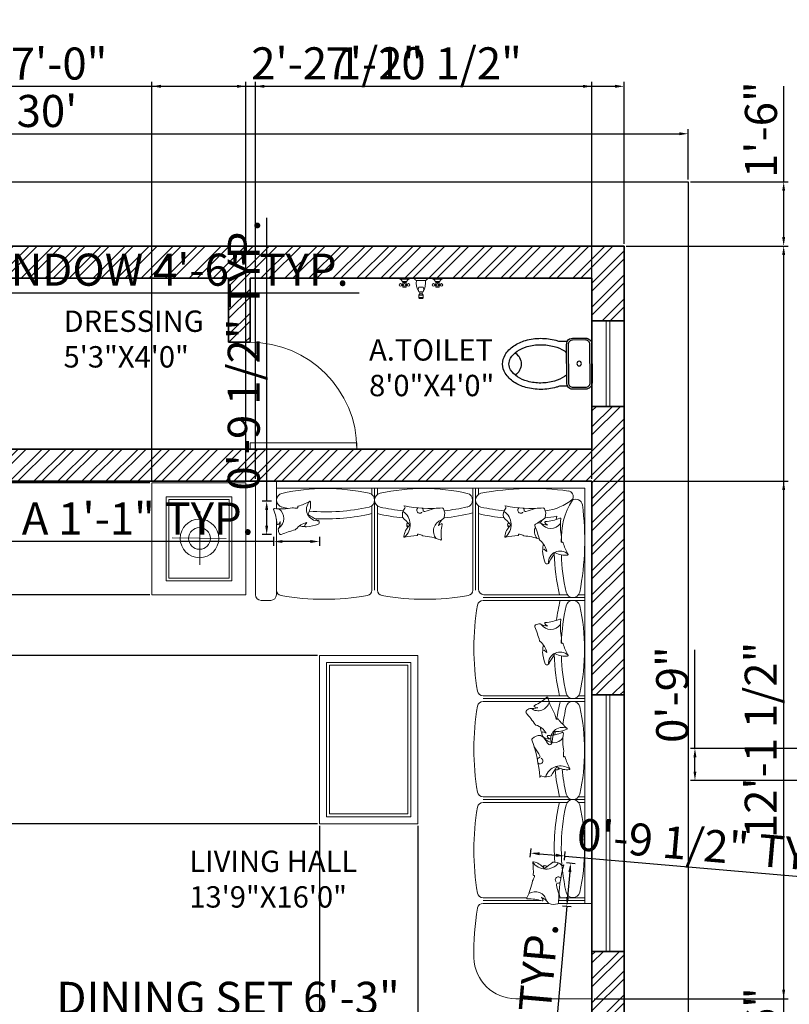
# Model space of a CAD drawing. Units: inches. Extents: x 638 to 1853, y 4393 to 5041.
# Tile 3 of 6: x 856 to 1072, y 4693 to 4970. Entities that reach past the tile are written whole.
import ezdxf

# ---------------------------------------------------------------- set-up
doc = ezdxf.new("R2010")
doc.units = ezdxf.units.IN
for name, color, linetype, lineweight in [('A-ANNO-DIMS', 2, 'Continuous', 18), ('A-AREA-IDEN', 7, 'Continuous', 18), ('A-DOOR', 4, 'Continuous', 18), ('A-FLOR-FIXT', 9, 'Continuous', 18), ('A-FURN', 26, 'Continuous', 13), ('A-GLAZ', 5, 'Continuous', 18), ('A-WALL', 7, 'Continuous', 35), ('A-WALL-PATT', 251, 'Continuous', 13), ('C-PROP', 7, 'Continuous', 25)]:
    doc.layers.add(name, color=color, linetype=linetype, lineweight=lineweight)
doc.layers.add('SANTEH', color=7, linetype='Continuous')
doc.styles.get("Standard").update_dxf_attribs({"font": 'arial.ttf'})
doc.dimstyles.new('ISO-25', dxfattribs={"dimtxt": 9, "dimasz": 2.5, "dimexe": 1.25, "dimexo": 0.625, "dimtad": 1, "dimdec": 1, "dimlunit": 3, "dimtxsty": 'Standard', "dimcen": 2.5, "dimadec": 0, "dimazin": 0, "dimtfac": 1, "dimtdec": 1, "dimtmove": 0, "dimatfit": 3, "dimfxl": 1, "dimarcsym": 0})

# ---------------------------------------------------------------- blocks, each defined once
blk = doc.blocks.new('*U3')
for p, q in [((-30, 0), (-30, -6)), ((0, 0), (0, -6))]:
    blk.add_line(p, q)
blk.add_lwpolyline([(0, 0), (0, 30), (-1.75, 30), (-1.75, 0)], close=True)
blk.add_arc((0, 0), 30, 90, 180)
blk = doc.blocks.new('K10-44')
at = {"layer": 'SANTEH'}
for points in [[(-182, 222.6, 0.020439), (-174, 197.6), (-174, 134.8, 0.262987), (-198.2, 92), (-198.2, -8, 0.414214), (-148.2, -58), (151.8, -58, 0.414214), (201.8, -8), (201.8, 92, 0.262987), (177.6, 134.8), (177.6, 197.6, 0.020439), (185.6, 222.6, 0.067459), (201.8, 342, 0.067459), (185.6, 461.3, 0.079812), (143.2, 554.1, 0.107118), (73.7, 621.5, 0.139889), (1.8, 642, 0.139889), (-70.1, 621.5, 0.107118), (-139.6, 554.1, 0.079812), (-182, 461.3, 0.067459), (-198.2, 342, 0.067459)], [(-148.2, 127), (151.8, 127, -0.414214), (186.8, 92), (186.8, -8, -0.414214), (151.8, -43), (-148.2, -43, -0.414214), (-183.2, -8), (-183.2, 92, -0.414214)]]:
    blk.add_lwpolyline(points, format="xyb", close=True, dxfattribs=at)
for points in [[(89.9, 142, 0.027307), (101.6, 157.6, 0.079812), (137.4, 235.9, 0.067459), (151.8, 342, 0.067459), (137.4, 448, 0.079812), (101.6, 526.4, 0.107118), (47.3, 579, 0.139889), (1.8, 592, 0.139889), (-43.7, 579, 0.107118), (-98, 526.4, 0.079812), (-133.8, 448, 0.067459), (-148.2, 342, 0.067459), (-133.8, 235.9, 0.079812), (-98, 157.6, 0.027307), (-86.4, 142, 0.139889)], [(-174, 134.8, -0.136371), (-148.2, 142), (151.8, 142, -0.136371), (177.6, 134.8)]]:
    blk.add_lwpolyline(points, format="xyb", dxfattribs=at)
blk.add_circle((1.8, 42), 18.3, dxfattribs=at)
blk.add_arc((1.8, 601.6), 105.3, 213.89944, 326.10056, dxfattribs=at)
blk = doc.blocks.new('Faucet - Bathroom front')
for p, q in [((-0.5, 4.25), (0.5, 4.25)), ((0.5, 3.75), (-0.5, 3.75)), ((-0.5, 3), (0.5, 3)), ((-0.25, 3), (-0.25, 3.5)), ((0.25, 3.5), (0.25, 3)), ((-5, 0), (-2.25, 0)), ((-4.5087, 0.25), (-2.7408, 0.25)), ((-4, 1.625), (-4.25, 1.625)), ((-4, 1.375), (-4.25, 1.375)), ((-3.1442, 0.75), (-4.0979, 0.75)), ((-3.25, 1.625), (-3, 1.625)), ((-3.25, 1.375), (-3, 1.375)), ((-1.5, 0), (1.5, 0)), ((-1, 0.5), (1, 0.5)), ((0.5, 2), (-0.5, 2)), ((2.25, 0), (5, 0)), ((2.7413, 0.25), (4.5092, 0.25)), ((3.25, 1.625), (3, 1.625)), ((3.25, 1.375), (3, 1.375)), ((4.1058, 0.75), (3.1521, 0.75)), ((4, 1.625), (4.25, 1.625)), ((4, 1.375), (4.25, 1.375))]:
    blk.add_line(p, q)
for points in [[(-0.25, 4.5), (0.25, 4.5)], [(-0.5, 3.75), (-0.5, 4.25)], [(0.25, 3.5), (-0.25, 3.5)], [(0.5, 4.25), (0.5, 3.75)]]:
    blk.add_lwpolyline(points)
for points in [[(-4, 1), (-4, 2), (-3.25, 2), (-3.25, 1)], [(3.25, 1), (3.25, 2), (4, 2), (4, 1)]]:
    blk.add_lwpolyline(points, close=True)
for centre in [(-4.5, 1.5), (-3.625, 1.5), (-2.75, 1.5), (2.75, 1.5), (3.625, 1.5), (4.5, 1.5)]:
    blk.add_circle(centre, 0.2795)
for centre, radius, start, end in [((-0.2575, 4.2575), 0.2426, 88.22243, 181.7776), ((0.2575, 4.2575), 0.2426, 358.2224, 91.77757), ((3, 1), 4.0311, 150.2551, 187.125), ((0.6413, 2.5), 1.246, 156.3417, 203.6583), ((-0.2575, 3.7425), 0.2426, 178.2224, 271.7776), ((0.2575, 3.7425), 0.2426, 268.2224, 1.777565), ((-3, 1), 4.0311, 352.875, 29.74488), ((-0.6413, 2.5), 1.246, 336.3417, 23.65835), ((-5.375, 1.375), 1.4252, 285.2551, 344.7449), ((-1.875, 1.375), 1.4252, 195.2551, 254.7449), ((-0.7962, -0.2038), 0.7327, 106.1502, 163.8498), ((0.7962, -0.2038), 0.7327, 16.1502, 73.84979), ((1.875, 1.375), 1.4252, 285.2551, 344.7449), ((5.375, 1.375), 1.4252, 195.2551, 254.7449)]:
    blk.add_arc(centre, radius, start, end)
blk = doc.blocks.new('*D16')
at = {"layer": 'A-ANNO-DIMS', "color": 0, "lineweight": -2, "transparency": 16777216}
for p, q in [((683.34, 4924.82), (683.34, 4938.95)), ((1043.34, 4924.82), (1043.34, 4938.95)), ((685.84, 4937.7), (1040.84, 4937.7))]:
    blk.add_line(p, q, dxfattribs=at)
at = {"layer": 'A-ANNO-DIMS', "color": 0, "transparency": 16777216}
for points in [[(685.84, 4938.12), (685.84, 4937.29), (683.34, 4937.7)], [(1040.84, 4938.12), (1040.84, 4937.29), (1043.34, 4937.7)]]:
    blk.add_solid(points, dxfattribs=at)
at = {"layer": 'Defpoints', "color": 0, "transparency": 16777216}
for p in [(1043.34, 4937.7), (683.34, 4924.19), (1043.34, 4924.19)]:
    blk.add_point(p, dxfattribs=at)
at = {"layer": 'A-ANNO-DIMS', "color": 0, "transparency": 16777216, "insert": (863.34, 4942.93), "char_height": 9, "attachment_point": 5}
blk.add_mtext("30'", dxfattribs=at)
blk = doc.blocks.new('SOFA-THROW-PILLOW-A')
for centre, radius, start, end in [((0.39, 10.82), 0.394, 117.1304, 200.9482), ((1.62, 8.42), 3.09, 92.7962, 117.1304), ((3.55, 15.03), 4.09, 239.5087, 271.0429), ((4.49, 13.18), 3.27, 214.0212, 325.1506), ((2.96, 11.66), 0.197, 93.9947, 209.557), ((3.91, 12.2), 1.3, 209.557, 257.0475), ((2.03, 24.94), 13.11, 273.9947, 292.2174), ((7.06, 12.62), 0.197, 353.9832, 112.2174), ((23.64, 10.87), 16.48, 173.9832, 191.5286), ((-38.21, -3.96), 40.94, 15.1521, 20.9482), ((1.69, 6.84), 0.394, 195.1521, 232.4345), ((-1.66, 2.48), 5.11, 10.921, 52.4345), ((10.08, 4.04), 7.86, 168.5381, 180.9308), ((15.26, 6.3), 7.86, 170.6752, 180.5669), ((7.59, 6.23), 0.197, 180.5669, 291.9475), ((7.74, 5.86), 0.197, 17.478, 111.9475), ((23.64, 10.87), 16.48, 197.478, 209.4698), ((2.54, 3.69), 0.394, 41.4659, 190.4525), ((16.93, 5.2), 14.87, 186.1256, 199.3393), ((6.12, 6.85), 4.39, 221.4659, 230.8131), ((7.05, 0.33), 3.25, 45.6927, 183.5175), ((38.1, -18.02), 38.77, 147.1103, 151.1368), ((5.7, 2.93), 0.197, 60.4242, 147.1103), ((8.39, 7.66), 5.25, 240.4242, 278.3824), ((3.28, 0.41), 0.394, 199.3393, 253.8009), ((3.38, 0.76), 0.764, 253.8009, 355.0524), ((9.13, 2.67), 0.197, 278.3824, 29.4698)]:
    blk.add_arc(centre, radius, start, end)
blk = doc.blocks.new('SOFA-THROW-PILLOW-B')
for centre, radius, start, end in [((3.19, 7), 3.19, 142.1663, 190.7613), ((0.36, 9.2), 0.394, 322.1663, 79.3422), ((8, 49.83), 40.94, 259.5852, 274.4465), ((4.89, 8.38), 0.833, 127.3565, 320.7762), ((4.94, 8.37), 0.873, 7.7015, 42.1556), ((5.42, 8.43), 0.394, 357.6426, 7.7015), ((6.2, 8.4), 0.394, 177.6426, 284.049), ((1.87, 25.7), 18.23, 284.049, 292.3823), ((9, 8.5), 0.394, 91.386, 118.7955), ((8, 49.83), 40.94, 271.386, 274.4465), ((11.21, 8.61), 0.394, 26.666, 94.4465), ((8.69, 7.35), 3.21, 342.3377, 26.666), ((-27.35, -21.02), 38.77, 40.8329, 45.0245), ((-2.23, 4.27), 4.44, 308.8947, 57.3952), ((12.01, 2.51), 3.27, 107.7628, 218.8922), ((14.05, 2.89), 4.09, 126.6071, 164.7845), ((11.38, 6.49), 0.394, 306.6071, 342.3377), ((5.62, 0.31), 5.25, 134.9211, 172.124), ((2, 4.24), 0.787, 127.662, 234.1573), ((15.2, 45.86), 44.04, 251.4982, 252.2888), ((7.81, -38.62), 44.04, 97.7018, 97.7206), ((1.84, 4.2), 0.197, 293.8315, 40.8329), ((11.24, 3.33), 1.3, 103.2985, 150.7891), ((23.99, 1.58), 13.11, 167.7363, 185.959), ((10.98, 4.41), 0.197, 347.7363, 103.2985), ((0.62, 1), 0.197, 172.124, 283.2114), ((0.62, 1), 0.197, 172.124, 283.2114), ((4.43, -15.23), 16.48, 91.2196, 103.2114), ((4.08, 1.44), 0.197, 271.2196, 5.689), ((4.47, 1.48), 0.197, 74.3085, 185.689), ((2.4, -5.9), 7.86, 64.4168, 74.3085), ((4.43, -15.23), 16.48, 67.7248, 85.2702), ((10.75, 0.2), 0.197, 247.7248, 5.959)]:
    blk.add_arc(centre, radius, start, end)
blk = doc.blocks.new('WINDOW-GLAZING-24IN')
for p, q in [((0, 24), (0, 0)), ((1, 24), (1, 0))]:
    blk.add_line(p, q)
blk = doc.blocks.new('WINDOW-GLAZING-72IN')
for p, q in [((0, 72), (0, 0)), ((1, 72), (1, 0))]:
    blk.add_line(p, q)
blk = doc.blocks.new('*D44')
at = {"layer": 'A-ANNO-DIMS', "color": 0, "lineweight": -2, "transparency": 16777216}
for p, q in [((926.95, 4823.26), (805.91, 4823.26)), ((926.95, 4824.56), (926.95, 4822.01)), ((937.31, 4823.26), (929.45, 4823.26)), ((939.81, 4824.56), (939.81, 4822.01))]:
    blk.add_line(p, q, dxfattribs=at)
at = {"layer": 'A-ANNO-DIMS', "color": 0, "transparency": 16777216}
for points in [[(929.45, 4823.67), (929.45, 4822.84), (926.95, 4823.26)], [(937.31, 4823.67), (937.31, 4822.84), (939.81, 4823.26)]]:
    blk.add_solid(points, dxfattribs=at)
at = {"layer": 'Defpoints', "color": 0, "transparency": 16777216}
for p in [(926.95, 4825.19), (926.95, 4823.26), (939.81, 4825.19)]:
    blk.add_point(p, dxfattribs=at)
at = {"layer": 'A-ANNO-DIMS', "color": 0, "transparency": 16777216, "insert": (865.18, 4828.54), "char_height": 9, "attachment_point": 5}
blk.add_mtext('PILLOW A 1\'-1" TYP.', dxfattribs=at)
blk = doc.blocks.new('*D45')
at = {"layer": 'A-ANNO-DIMS', "color": 0, "lineweight": -2, "transparency": 16777216}
for p, q in [((925.02, 4834.56), (925.02, 4914.14)), ((926.33, 4834.56), (923.77, 4834.56)), ((925.02, 4827.69), (925.02, 4832.06)), ((926.33, 4825.19), (923.77, 4825.19))]:
    blk.add_line(p, q, dxfattribs=at)
at = {"layer": 'A-ANNO-DIMS', "color": 0, "transparency": 16777216}
for points in [[(924.61, 4832.06), (925.44, 4832.06), (925.02, 4834.56)], [(924.61, 4827.69), (925.44, 4827.69), (925.02, 4825.19)]]:
    blk.add_solid(points, dxfattribs=at)
at = {"layer": 'Defpoints', "color": 0, "transparency": 16777216}
for p in [(925.02, 4834.56), (926.95, 4834.56), (926.95, 4825.19)]:
    blk.add_point(p, dxfattribs=at)
at = {"layer": 'A-ANNO-DIMS', "color": 0, "transparency": 16777216, "insert": (919.75, 4875.6), "char_height": 9, "attachment_point": 5, "rotation": 90}
blk.add_mtext('0\'-9 1/2" TYP.', dxfattribs=at)
blk = doc.blocks.new('*D46')
at = {"layer": 'A-ANNO-DIMS', "color": 0, "lineweight": -2, "transparency": 16777216}
for p, q in [((779.34, 4900.57), (779.34, 4891.84)), ((833.34, 4900.57), (833.34, 4891.84)), ((781.84, 4893.09), (830.84, 4893.09)), ((833.34, 4893.09), (950.98, 4893.09))]:
    blk.add_line(p, q, dxfattribs=at)
at = {"layer": 'A-ANNO-DIMS', "color": 0, "transparency": 16777216}
for points in [[(781.84, 4893.51), (781.84, 4892.68), (779.34, 4893.09)], [(830.84, 4893.51), (830.84, 4892.68), (833.34, 4893.09)]]:
    blk.add_solid(points, dxfattribs=at)
at = {"layer": 'Defpoints', "color": 0, "transparency": 16777216}
for p in [(779.34, 4901.19), (833.34, 4901.19), (833.34, 4893.09)]:
    blk.add_point(p, dxfattribs=at)
at = {"layer": 'A-ANNO-DIMS', "color": 0, "transparency": 16777216, "insert": (893.41, 4898.38), "char_height": 9, "attachment_point": 5}
blk.add_mtext('WINDOW 4\'-6" TYP.', dxfattribs=at)
blk = doc.blocks.new('*D50')
at = {"layer": 'A-ANNO-DIMS', "color": 0, "lineweight": -2, "transparency": 16777216}
for p, q in [((1009.16, 4733.11), (1011.59, 4732.9)), ((1010.13, 4730.52), (1009.51, 4723.42)), ((1009.29, 4720.93), (998.74, 4600.35)), ((1008.1, 4721.03), (1010.54, 4720.82))]:
    blk.add_line(p, q, dxfattribs=at)
at = {"layer": 'A-ANNO-DIMS', "color": 0, "transparency": 16777216}
for points in [[(1009.71, 4730.55), (1010.54, 4730.48), (1010.35, 4733.01)], [(1009.09, 4723.46), (1009.92, 4723.38), (1009.29, 4720.93)]]:
    blk.add_solid(points, dxfattribs=at)
at = {"layer": 'Defpoints', "color": 0, "transparency": 16777216}
for p in [(1008.54, 4733.16), (1007.48, 4721.09), (1009.29, 4720.93)]:
    blk.add_point(p, dxfattribs=at)
at = {"layer": 'A-ANNO-DIMS', "color": 0, "transparency": 16777216, "insert": (998.65, 4659.85), "char_height": 9, "attachment_point": 5, "rotation": 85}
blk.add_mtext('PILLOW B 1\'-0" TYP.', dxfattribs=at)
blk = doc.blocks.new('*D51')
at = {"layer": 'A-ANNO-DIMS', "color": 0, "lineweight": -2, "transparency": 16777216}
for p, q in [((999.03, 4734.62), (999.24, 4737.06)), ((1001.62, 4735.59), (1006.2, 4735.19)), ((1008.59, 4733.79), (1008.8, 4736.22)), ((1008.69, 4734.98), (1087.97, 4728.04))]:
    blk.add_line(p, q, dxfattribs=at)
at = {"layer": 'A-ANNO-DIMS', "color": 0, "transparency": 16777216}
for points in [[(1001.66, 4736.01), (1001.59, 4735.18), (999.13, 4735.81)], [(1006.24, 4735.61), (1006.17, 4734.78), (1008.69, 4734.98)]]:
    blk.add_solid(points, dxfattribs=at)
at = {"layer": 'Defpoints', "color": 0, "transparency": 16777216}
for p in [(1008.69, 4734.98), (998.97, 4734), (1008.54, 4733.16)]:
    blk.add_point(p, dxfattribs=at)
at = {"layer": 'A-ANNO-DIMS', "color": 0, "transparency": 16777216, "insert": (1050.04, 4736.66), "char_height": 9, "attachment_point": 5, "rotation": 355}
blk.add_mtext('0\'-9 1/2" TYP.', dxfattribs=at)
blk = doc.blocks.new('*D62')
at = {"layer": 'A-ANNO-DIMS', "color": 0, "lineweight": -2, "transparency": 16777216}
for p, q in [((786.73, 4678.11), (786.73, 4689.96)), ((861.6, 4678.11), (861.6, 4689.96)), ((789.23, 4688.71), (859.1, 4688.71)), ((861.6, 4688.71), (964.27, 4688.71))]:
    blk.add_line(p, q, dxfattribs=at)
at = {"layer": 'A-ANNO-DIMS', "color": 0, "transparency": 16777216}
for points in [[(789.23, 4689.13), (789.23, 4688.3), (786.73, 4688.71)], [(859.1, 4689.13), (859.1, 4688.3), (861.6, 4688.71)]]:
    blk.add_solid(points, dxfattribs=at)
at = {"layer": 'Defpoints', "color": 0, "transparency": 16777216}
for p in [(861.6, 4688.71), (786.73, 4677.48), (861.6, 4677.48)]:
    blk.add_point(p, dxfattribs=at)
at = {"layer": 'A-ANNO-DIMS', "color": 0, "transparency": 16777216, "insert": (914.18, 4694), "char_height": 9, "attachment_point": 5}
blk.add_mtext('DINING SET 6\'-3"', dxfattribs=at)
blk = doc.blocks.new('*D74')
at = {"layer": 'A-ANNO-DIMS', "color": 0, "lineweight": -2, "transparency": 16777216}
for p, q in [((701.34, 4906.82), (701.34, 4952.27)), ((703.84, 4951.02), (1022.84, 4951.02)), ((1025.34, 4906.82), (1025.34, 4952.27))]:
    blk.add_line(p, q, dxfattribs=at)
at = {"layer": 'A-ANNO-DIMS', "color": 0, "transparency": 16777216}
for points in [[(703.84, 4951.44), (703.84, 4950.6), (701.34, 4951.02)], [(1022.84, 4951.44), (1022.84, 4950.6), (1025.34, 4951.02)]]:
    blk.add_solid(points, dxfattribs=at)
at = {"layer": 'Defpoints', "color": 0, "transparency": 16777216}
for p in [(1025.34, 4951.02), (701.34, 4906.19), (1025.34, 4906.19)]:
    blk.add_point(p, dxfattribs=at)
at = {"layer": 'A-ANNO-DIMS', "color": 0, "transparency": 16777216, "insert": (863.34, 4956.24), "char_height": 9, "attachment_point": 5}
blk.add_mtext('27\'-0"', dxfattribs=at)
blk = doc.blocks.new('*D75')
at = {"layer": 'A-ANNO-DIMS', "color": 0, "lineweight": -2, "transparency": 16777216}
for p, q in [((1025.97, 4906.19), (1071.42, 4906.19)), ((1070.17, 4458.69), (1070.17, 4903.69)), ((896.97, 4456.19), (1071.42, 4456.19))]:
    blk.add_line(p, q, dxfattribs=at)
at = {"layer": 'A-ANNO-DIMS', "color": 0, "transparency": 16777216}
for points in [[(1069.75, 4903.69), (1070.58, 4903.69), (1070.17, 4906.19)], [(1069.75, 4458.69), (1070.58, 4458.69), (1070.17, 4456.19)]]:
    blk.add_solid(points, dxfattribs=at)
at = {"layer": 'Defpoints', "color": 0, "transparency": 16777216}
for p in [(1025.34, 4906.19), (1070.17, 4906.19), (896.34, 4456.19)]:
    blk.add_point(p, dxfattribs=at)
at = {"layer": 'A-ANNO-DIMS', "color": 0, "transparency": 16777216, "insert": (1064.94, 4681.19), "char_height": 9, "attachment_point": 5, "rotation": 90}
blk.add_mtext('37\'-6"', dxfattribs=at)
blk = doc.blocks.new('*D77')
at = {"layer": 'A-ANNO-DIMS', "color": 0, "lineweight": -2, "transparency": 16777216}
for p, q in [((1070.17, 4924.19), (1070.17, 4951.02)), ((1043.97, 4924.19), (1071.42, 4924.19)), ((1070.17, 4908.69), (1070.17, 4921.69)), ((1025.97, 4906.19), (1071.42, 4906.19))]:
    blk.add_line(p, q, dxfattribs=at)
at = {"layer": 'A-ANNO-DIMS', "color": 0, "transparency": 16777216}
for points in [[(1069.75, 4921.69), (1070.58, 4921.69), (1070.17, 4924.19)], [(1069.75, 4908.69), (1070.58, 4908.69), (1070.17, 4906.19)]]:
    blk.add_solid(points, dxfattribs=at)
at = {"layer": 'Defpoints', "color": 0, "transparency": 16777216}
for p in [(1043.34, 4924.19), (1070.17, 4924.19), (1025.34, 4906.19)]:
    blk.add_point(p, dxfattribs=at)
at = {"layer": 'A-ANNO-DIMS', "color": 0, "transparency": 16777216, "insert": (1064.95, 4938.86), "char_height": 9, "attachment_point": 5, "rotation": 90}
blk.add_mtext('1\'-6"', dxfattribs=at)
blk = doc.blocks.new('*D82')
at = {"layer": 'A-ANNO-DIMS', "color": 0, "lineweight": -2, "transparency": 16777216}
for p, q in [((921.85, 4840.82), (921.85, 4952.27)), ((924.35, 4951.02), (1013.84, 4951.02)), ((1016.34, 4840.82), (1016.34, 4952.27))]:
    blk.add_line(p, q, dxfattribs=at)
at = {"layer": 'A-ANNO-DIMS', "color": 0, "transparency": 16777216}
for points in [[(924.35, 4951.44), (924.35, 4950.6), (921.85, 4951.02)], [(1013.84, 4951.44), (1013.84, 4950.6), (1016.34, 4951.02)]]:
    blk.add_solid(points, dxfattribs=at)
at = {"layer": 'Defpoints', "color": 0, "transparency": 16777216}
for p in [(1016.34, 4951.02), (921.85, 4840.19), (1016.34, 4840.19)]:
    blk.add_point(p, dxfattribs=at)
at = {"layer": 'A-ANNO-DIMS', "color": 0, "transparency": 16777216, "insert": (969.1, 4956.3), "char_height": 9, "attachment_point": 5}
blk.add_mtext('7\'-10 1/2"', dxfattribs=at)
blk = doc.blocks.new('*D83')
at = {"layer": 'A-ANNO-DIMS', "color": 0, "lineweight": -2, "transparency": 16777216}
for p, q in [((1016.97, 4840.19), (1071.42, 4840.19)), ((1070.17, 4697.42), (1070.17, 4837.69)), ((1016.97, 4694.92), (1071.42, 4694.92))]:
    blk.add_line(p, q, dxfattribs=at)
at = {"layer": 'A-ANNO-DIMS', "color": 0, "transparency": 16777216}
for points in [[(1069.75, 4837.69), (1070.58, 4837.69), (1070.17, 4840.19)], [(1069.75, 4697.42), (1070.58, 4697.42), (1070.17, 4694.92)]]:
    blk.add_solid(points, dxfattribs=at)
at = {"layer": 'Defpoints', "color": 0, "transparency": 16777216}
for p in [(1016.34, 4840.19), (1070.17, 4840.19), (1016.34, 4694.92)]:
    blk.add_point(p, dxfattribs=at)
at = {"layer": 'A-ANNO-DIMS', "color": 0, "transparency": 16777216, "insert": (1064.89, 4767.56), "char_height": 9, "attachment_point": 5, "rotation": 90}
blk.add_mtext('12\'-1 1/2"', dxfattribs=at)
blk = doc.blocks.new('*D84')
at = {"layer": 'A-ANNO-DIMS', "color": 0, "lineweight": -2, "transparency": 16777216}
for p, q in [((939.87, 4743.42), (939.87, 4416.12)), ((967.43, 4743.42), (967.43, 4416.12)), ((942.37, 4417.37), (964.93, 4417.37)), ((967.43, 4417.37), (1016.23, 4417.37))]:
    blk.add_line(p, q, dxfattribs=at)
at = {"layer": 'A-ANNO-DIMS', "color": 0, "transparency": 16777216}
for points in [[(942.37, 4417.79), (942.37, 4416.95), (939.87, 4417.37)], [(964.93, 4417.79), (964.93, 4416.95), (967.43, 4417.37)]]:
    blk.add_solid(points, dxfattribs=at)
at = {"layer": 'Defpoints', "color": 0, "transparency": 16777216}
for p in [(939.87, 4744.04), (967.43, 4744.04), (967.43, 4417.37)]:
    blk.add_point(p, dxfattribs=at)
at = {"layer": 'A-ANNO-DIMS', "color": 0, "transparency": 16777216, "insert": (993.08, 4422.65), "char_height": 9, "attachment_point": 5}
blk.add_mtext('2\'-3 1/2"', dxfattribs=at)
blk = doc.blocks.new('*D85')
at = {"layer": 'A-ANNO-DIMS', "color": 0, "lineweight": -2, "transparency": 16777216}
for p, q in [((939.25, 4791.29), (655.27, 4791.29)), ((656.52, 4746.54), (656.52, 4788.79)), ((939.25, 4744.04), (655.27, 4744.04))]:
    blk.add_line(p, q, dxfattribs=at)
at = {"layer": 'A-ANNO-DIMS', "color": 0, "transparency": 16777216}
for points in [[(656.1, 4788.79), (656.93, 4788.79), (656.52, 4791.29)], [(656.1, 4746.54), (656.93, 4746.54), (656.52, 4744.04)]]:
    blk.add_solid(points, dxfattribs=at)
at = {"layer": 'Defpoints', "color": 0, "transparency": 16777216}
for p in [(656.52, 4791.29), (939.87, 4791.29), (939.87, 4744.04)]:
    blk.add_point(p, dxfattribs=at)
at = {"layer": 'A-ANNO-DIMS', "color": 0, "transparency": 16777216, "insert": (651.29, 4767.66), "char_height": 9, "attachment_point": 5, "rotation": 90}
blk.add_mtext('3\'-11"', dxfattribs=at)
blk = doc.blocks.new('*D86')
at = {"layer": 'A-ANNO-DIMS', "color": 0, "lineweight": -2, "transparency": 16777216}
for p, q in [((892.82, 4840.37), (892.82, 4952.27)), ((895.32, 4951.02), (916.69, 4951.02)), ((919.19, 4840.37), (919.19, 4952.27)), ((919.19, 4951.02), (967.99, 4951.02))]:
    blk.add_line(p, q, dxfattribs=at)
at = {"layer": 'A-ANNO-DIMS', "color": 0, "transparency": 16777216}
for points in [[(895.32, 4951.44), (895.32, 4950.6), (892.82, 4951.02)], [(916.69, 4951.44), (916.69, 4950.6), (919.19, 4951.02)]]:
    blk.add_solid(points, dxfattribs=at)
at = {"layer": 'Defpoints', "color": 0, "transparency": 16777216}
for p in [(919.19, 4951.02), (892.82, 4839.74), (919.19, 4839.74)]:
    blk.add_point(p, dxfattribs=at)
at = {"layer": 'A-ANNO-DIMS', "color": 0, "transparency": 16777216, "insert": (944.84, 4956.3), "char_height": 9, "attachment_point": 5}
blk.add_mtext('2\'-2 1/2"', dxfattribs=at)
blk = doc.blocks.new('*D87')
at = {"layer": 'A-ANNO-DIMS', "color": 0, "lineweight": -2, "transparency": 16777216}
for p, q in [((656.52, 4839.74), (656.52, 4888.54)), ((892.19, 4839.74), (655.27, 4839.74)), ((656.52, 4810.75), (656.52, 4837.24)), ((892.19, 4808.25), (655.27, 4808.25))]:
    blk.add_line(p, q, dxfattribs=at)
at = {"layer": 'A-ANNO-DIMS', "color": 0, "transparency": 16777216}
for points in [[(656.1, 4837.24), (656.93, 4837.24), (656.52, 4839.74)], [(656.1, 4810.75), (656.93, 4810.75), (656.52, 4808.25)]]:
    blk.add_solid(points, dxfattribs=at)
at = {"layer": 'Defpoints', "color": 0, "transparency": 16777216}
for p in [(656.52, 4839.74), (892.82, 4839.74), (892.82, 4808.25)]:
    blk.add_point(p, dxfattribs=at)
at = {"layer": 'A-ANNO-DIMS', "color": 0, "transparency": 16777216, "insert": (651.24, 4865.39), "char_height": 9, "attachment_point": 5, "rotation": 90}
blk.add_mtext('2\'-7 1/2"', dxfattribs=at)
blk = doc.blocks.new('*D93')
at = {"layer": 'A-ANNO-DIMS', "color": 0, "lineweight": -2, "transparency": 16777216}
for p, q in [((1045.26, 4765.19), (1045.26, 4792.87)), ((1284.46, 4765.19), (1044.01, 4765.19)), ((1045.26, 4758.69), (1045.26, 4762.69)), ((1275.46, 4756.19), (1044.01, 4756.19))]:
    blk.add_line(p, q, dxfattribs=at)
at = {"layer": 'A-ANNO-DIMS', "color": 0, "transparency": 16777216}
for points in [[(1044.84, 4762.69), (1045.67, 4762.69), (1045.26, 4765.19)], [(1044.84, 4758.69), (1045.67, 4758.69), (1045.26, 4756.19)]]:
    blk.add_solid(points, dxfattribs=at)
at = {"layer": 'Defpoints', "color": 0, "transparency": 16777216}
for p in [(1045.26, 4765.19), (1285.08, 4765.19), (1276.08, 4756.19)]:
    blk.add_point(p, dxfattribs=at)
at = {"layer": 'A-ANNO-DIMS', "color": 0, "transparency": 16777216, "insert": (1040.04, 4780.28), "char_height": 9, "attachment_point": 5, "rotation": 90}
blk.add_mtext('0\'-9"', dxfattribs=at)

msp = doc.modelspace()

# ---------------------------------------------------------------- hatches: boundary and pattern name
at = {"layer": 'A-WALL-PATT', "transparency": 33554687}
h = msp.add_hatch(dxfattribs=at)
h.set_pattern_fill('ANSI32', color=256, scale=0.5)
h.paths.add_polyline_path([(779.34, 4906.19), (701.34, 4906.19), (701.34, 4531.19), (710.34, 4531.19), (710.34, 4561.19), (758.34, 4561.19), (758.34, 4528.19), (764.34, 4528.19), (767.34, 4528.19), (767.34, 4561.19), (821.34, 4561.19), (821.34, 4570.19), (710.34, 4570.19), (710.34, 4756.19), (767.34, 4756.19), (767.34, 4702.19), (791.34, 4702.19), (791.34, 4708.19), (773.34, 4708.19), (773.34, 4756.19), (845.34, 4756.19), (845.34, 4708.19), (827.35, 4708.19), (827.35, 4705.02), (827.34, 4702.19), (851.34, 4702.19), (851.34, 4771.19), (845.34, 4771.19), (842.34, 4771.19), (842.34, 4765.19), (710.34, 4765.19), (710.34, 4897.19), (779.34, 4897.19)])
h.paths.add_polyline_path([(1025.34, 4906.19), (833.34, 4906.19), (833.34, 4897.19), (842.34, 4897.19), (842.34, 4882.21), (842.34, 4879.19), (851.34, 4879.19), (851.34, 4897.19), (914.34, 4897.19), (914.34, 4879.19), (920.34, 4879.19), (920.34, 4897.19), (1016.34, 4897.19), (1016.34, 4885.19), (1025.34, 4885.19)])
h.paths.add_polyline_path([(851.34, 4840.19), (1016.34, 4840.19), (1016.34, 4780.19), (1025.34, 4780.19), (1025.34, 4861.19), (1016.34, 4861.19), (1016.34, 4849.19), (842.34, 4849.19), (842.34, 4807.19), (851.34, 4807.19)])
h.paths.add_polyline_path([(1025.34, 4708.19), (1016.34, 4708.19), (1016.34, 4694.92), (1016.34, 4648.19), (996.84, 4648.19), (996.84, 4639.19), (1025.34, 4639.19)])
h.paths.add_polyline_path([(972.84, 4648.19), (944.34, 4648.19), (944.34, 4561.19), (953.34, 4561.19), (953.34, 4639.19), (972.84, 4639.19)])
h.paths.add_polyline_path([(896.34, 4648.19), (887.34, 4648.19), (887.34, 4570.19), (863.34, 4570.19), (863.34, 4561.19), (887.34, 4561.19), (887.34, 4552.19), (896.34, 4552.19), (896.34, 4561.19), (904.34, 4561.19), (904.34, 4567.19), (904.34, 4570.19), (896.34, 4570.19)])
h.paths.add_polyline_path([(896.34, 4504.19), (887.34, 4504.19), (887.34, 4465.19), (839.34, 4465.19), (839.34, 4456.19), (896.34, 4456.19)])
h.paths.add_polyline_path([(779.34, 4465.19), (767.34, 4465.19), (767.34, 4498.19), (758.34, 4498.19), (758.34, 4465.19), (710.34, 4465.19), (710.34, 4495.19), (701.34, 4495.19), (701.34, 4456.19), (779.34, 4456.19)])
h.paths.add_polyline_path([(865.86, 4868.68), (912.64, 4868.68), (912.64, 4891.07), (865.86, 4891.07)], flags=9)
h.paths.add_polyline_path([(730.31, 4828.82), (807.82, 4828.82), (807.82, 4851.21), (730.31, 4851.21)], flags=25)

# ---------------------------------------------------------------- linework, layer by layer
at = {"layer": 'A-FURN'}
for p, q in [((921.85, 4840.19), (1016.34, 4840.19)), ((921.85, 4840.19), (921.85, 4808.31)), ((927.76, 4840.19), (927.76, 4832.44)), ((1016.34, 4694.92), (1016.34, 4840.19)), ((927.76, 4838.23), (1014.37, 4838.23)), ((954.53, 4838.23), (954.53, 4836.47)), ((955.32, 4838.23), (955.32, 4809.62)), ((956.1, 4838.23), (956.1, 4836.47)), ((982.88, 4838.23), (982.88, 4809.62)), ((983.66, 4838.23), (983.66, 4809.62)), ((984.45, 4838.23), (984.45, 4836.44)), ((1014.37, 4721.69), (1014.37, 4838.23)), ((906.24, 4831.76), (906.24, 4816.75)), ((954.53, 4833.24), (954.53, 4809.62)), ((956.1, 4833.24), (956.1, 4809.62)), ((984.45, 4833.27), (984.45, 4809.88)), ((927.76, 4829.51), (927.76, 4808.31)), ((898.53, 4824.3), (913.63, 4824.13)), ((923.43, 4806.73), (926.18, 4806.73)), ((1014.37, 4807.52), (985.77, 4807.52)), ((1014.37, 4806.73), (985.77, 4806.73)), ((1009.42, 4808.31), (986.03, 4808.31)), ((1014.37, 4808.31), (1012.58, 4808.31)), ((1009.39, 4779.96), (985.77, 4779.96)), ((1014.37, 4779.17), (985.77, 4779.17)), ((1014.37, 4778.38), (985.77, 4778.38)), ((1014.37, 4779.96), (1012.61, 4779.96)), ((1009.39, 4751.61), (985.77, 4751.61)), ((1014.37, 4750.82), (985.77, 4750.82)), ((1014.37, 4751.61), (1012.61, 4751.61)), ((1009.39, 4750.04), (985.77, 4750.04)), ((1014.37, 4750.04), (1012.61, 4750.04)), ((998.07, 4723.27), (985.77, 4723.27)), ((1014.37, 4723.27), (1007, 4723.27)), ((1001.99, 4722.48), (985.77, 4722.48)), ((1004.19, 4721.69), (985.77, 4721.69)), ((1016.34, 4721.69), (1006.86, 4721.69)), ((1014.37, 4722.48), (1006.98, 4722.48)), ((1016.34, 4694.92), (995.01, 4694.92))]:
    msp.add_line(p, q, dxfattribs=at)
for points in [[(892.82, 4808.25), (892.82, 4839.74), (919.19, 4839.74), (919.19, 4808.25)], [(896.76, 4812.19), (896.76, 4835.81), (915.25, 4835.81), (915.25, 4812.19)], [(897.54, 4812.97), (897.54, 4835.02), (914.46, 4835.02), (914.46, 4812.97)], [(939.87, 4791.29), (967.43, 4791.29), (967.43, 4744.04), (939.87, 4744.04)], [(941.84, 4789.32), (965.46, 4789.32), (965.46, 4746.01), (941.84, 4746.01)], [(942.63, 4788.53), (964.68, 4788.53), (964.68, 4746.8), (942.63, 4746.8)]]:
    msp.add_lwpolyline(points, close=True, dxfattribs=at)
for radius in [5.42, 3.06]:
    msp.add_circle((906.16, 4824.13), radius, dxfattribs=at)
for centre, radius, start, end in [((929.76, 4834.85), 1.97, 104.0803, 255.9197), ((941.58, 4781.92), 56.2, 77.4504, 102.6409), ((953.33, 4834.85), 1.98, 283.4421, 76.5579), ((957.3, 4834.85), 1.98, 103.4421, 256.5579), ((969.05, 4781.92), 56.2, 77.3591, 102.5496), ((980.87, 4834.85), 1.97, 284.0803, 75.9197), ((985.65, 4834.85), 1.98, 103.4421, 256.5579), ((999.36, 4764), 74.15, 81.9877, 101.0211), ((1009.53, 4835.88), 1.56, 333.697, 83.9411), ((1001.94, 4845.52), 13.69, 275.4659, 311.0389), ((1027.85, 4824.11), 20.11, 147.7546, 182.8868), ((1011.82, 4833.24), 1.88, 9.5129, 121.6132), ((941.58, 4887.78), 56.2, 257.3591, 259.3285), ((941.58, 4887.78), 56.2, 265.3473, 282.5496), ((941.58, 4887.78), 58.17, 266.9701, 282.8596), ((969.05, 4887.78), 58.17, 257.1404, 264.3693), ((969.05, 4887.78), 56.2, 257.4504, 264.1793), ((969.05, 4887.78), 58.17, 275.6604, 283.7486), ((969.05, 4887.78), 56.2, 275.9684, 282.6409), ((997.4, 4887.78), 58.17, 257.1404, 264.3693), ((997.4, 4887.78), 56.2, 257.4504, 264.1793), ((994.65, 4830.66), 3.19, 142.1663, 190.7613), ((989.23, 4827.93), 4.44, 308.8947, 57.3952), ((991.82, 4832.86), 0.394, 322.1663, 79.3422), ((999.47, 4873.49), 40.94, 259.5852, 274.4465), ((996.35, 4832.04), 0.833, 127.3565, 320.7762), ((996.4, 4832.03), 0.873, 7.7015, 42.1556), ((996.88, 4832.09), 0.394, 357.6426, 7.7015), ((997.66, 4832.06), 0.394, 177.6426, 284.049), ((993.34, 4849.36), 18.23, 284.049, 292.3823), ((1000.47, 4832.16), 0.394, 91.386, 118.7955), ((999.47, 4873.49), 40.94, 271.386, 274.4465), ((1002.67, 4832.27), 0.394, 26.666, 94.4465), ((1000.15, 4831.01), 3.21, 342.3377, 26.666), ((936.12, 4823.66), 78.19, 349.2257, 7.2701), ((964.11, 4802.64), 38.77, 40.8329, 45.0245), ((993.46, 4827.9), 0.787, 127.662, 234.1573), ((999.27, 4785.04), 44.04, 97.7018, 97.7206), ((1003.47, 4826.17), 3.27, 107.7628, 138.0745), ((1005.51, 4826.56), 4.09, 126.6071, 152.4764), ((1002.84, 4830.15), 0.394, 306.6071, 342.3377), ((997.4, 4887.78), 58.17, 275.6604, 278.9745), ((1063.93, 4821.25), 58.17, 171.0255, 171.9102), ((997.08, 4823.97), 5.25, 134.9211, 172.124), ((1006.66, 4869.52), 44.04, 251.4982, 252.2888), ((993.3, 4827.86), 0.197, 293.8315, 40.8329), ((1003.47, 4826.17), 3.27, 157.6246, 218.8922), ((992.08, 4824.66), 0.197, 172.124, 283.2114), ((992.08, 4824.66), 0.197, 172.124, 283.2114), ((995.89, 4808.43), 16.48, 91.2196, 103.2114), ((995.54, 4825.1), 0.197, 271.2196, 5.689), ((995.93, 4825.14), 0.197, 74.3085, 185.689), ((993.86, 4817.76), 7.86, 64.4168, 74.3085), ((995.89, 4808.43), 16.48, 69.7744, 85.2702), ((1063.93, 4821.25), 58.17, 181.3394, 192.8596), ((1063.93, 4821.25), 56.2, 181.7906, 192.5496), ((929.33, 4809.62), 1.57, 180, 260.2206), ((952.96, 4809.62), 1.57, 279.7794, 0), ((957.68, 4809.62), 1.57, 180, 260.2206), ((981.3, 4809.62), 1.57, 279.7794, 0), ((986.03, 4809.88), 1.57, 180, 270), ((1011, 4809.5), 1.98, 193.4421, 346.5579), ((923.43, 4808.31), 1.57, 180, 270), ((926.18, 4808.31), 1.57, 270, 0), ((941.14, 4878.14), 71.11, 260.2206, 279.7794), ((969.49, 4878.14), 71.11, 260.2206, 279.7794), ((985.77, 4805.16), 1.57, 90, 170.2206), ((1063.93, 4792.91), 58.17, 166.2514, 171.9102), ((1011, 4804.73), 1.97, 14.0803, 165.9197), ((1054.29, 4793.34), 71.11, 170.2206, 189.7794), ((1063.93, 4792.91), 56.2, 167.3591, 178.1165), ((958.07, 4792.91), 56.2, 347.4504, 12.6409), ((1063.93, 4792.91), 58.17, 181.3394, 192.8596), ((1063.93, 4792.91), 56.2, 181.7906, 192.5496), ((985.77, 4781.53), 1.57, 189.7794, 270), ((985.77, 4776.81), 1.57, 90, 170.2206), ((1063.93, 4764.56), 58.17, 166.2514, 171.2921), ((1011, 4781.15), 1.98, 193.4421, 346.5579), ((1054.29, 4765), 71.11, 170.2206, 189.7794), ((1063.93, 4764.56), 56.2, 167.3591, 172.5082), ((1011, 4776.38), 1.97, 14.0803, 165.9197), ((958.07, 4764.56), 56.2, 347.4504, 12.6409), ((1063.93, 4764.56), 58.17, 174.6528, 175.6154), ((1063.93, 4764.56), 56.2, 174.3658, 174.8718), ((1063.93, 4764.56), 58.17, 185.1856, 192.8596), ((1063.93, 4764.56), 56.2, 185.2768, 192.5496), ((985.77, 4753.19), 1.57, 189.7794, 270), ((1011, 4752.81), 1.98, 193.4421, 346.5579), ((1011, 4748.84), 1.98, 13.4421, 166.5579), ((1054.29, 4736.65), 71.11, 170.2206, 189.7794), ((985.77, 4748.46), 1.57, 90, 170.2206), ((1063.93, 4737.09), 58.17, 167.1404, 183.7557), ((1063.93, 4737.09), 56.2, 167.4504, 192.6409), ((958.07, 4737.09), 56.2, 347.3591, 12.5496), ((985.77, 4724.84), 1.57, 189.7794, 270), ((1063.93, 4737.09), 58.17, 192.2794, 193.7486), ((1011, 4725.27), 1.97, 194.0803, 345.9197), ((1054.29, 4708.3), 71.11, 170.2206, 181.5218), ((985.77, 4720.12), 1.57, 90, 170.2206), ((995.01, 4706.73), 11.81, 181.5218, 270)]:
    msp.add_arc(centre, radius, start, end, dxfattribs=at)
at = {"layer": 'A-WALL'}
for p, q in [((701.34, 4906.19), (1025.34, 4906.19)), ((1025.34, 4906.19), (1025.34, 4639.19)), ((851.34, 4897.19), (914.34, 4897.19)), ((914.34, 4897.19), (914.34, 4879.19)), ((920.34, 4897.19), (1016.34, 4897.19)), ((920.34, 4897.19), (920.34, 4879.19)), ((1016.34, 4897.19), (1016.34, 4849.19)), ((1016.34, 4885.19), (1025.34, 4885.19)), ((914.34, 4879.19), (920.34, 4879.19)), ((1016.34, 4861.19), (1025.34, 4861.19)), ((842.34, 4849.19), (1016.34, 4849.19)), ((851.34, 4840.19), (1016.34, 4840.19)), ((1016.34, 4840.19), (1016.34, 4648.19)), ((1016.34, 4780.19), (1025.34, 4780.19)), ((1016.34, 4708.19), (1025.34, 4708.19))]:
    msp.add_line(p, q, dxfattribs=at)
at = {"layer": 'C-PROP'}
msp.add_lwpolyline([(683.34, 4924.19), (1043.34, 4924.19), (1043.34, 4444.19), (683.34, 4444.19)], close=True, dxfattribs=at)

# ---------------------------------------------------------------- block references
at = {"layer": 'A-DOOR', "rotation": 270}
msp.add_blockref('*U3', (920.34, 4849.19), dxfattribs=at)
at = {"layer": 'A-FLOR-FIXT'}
for name, p, xscale, yscale, zscale, rotation in [('Faucet - Bathroom front', (968.34, 4897.19), 1.274234813154425, 1.274234813154425, 1.274234813154425, 180), ('K10-44', (1014.26, 4873.25), -0.0358529150226637, 0.0358529150226637, 0.0358529150226637, 90.3279556026283)]:
    msp.add_blockref(name, p, dxfattribs=dict(at, xscale=xscale, yscale=yscale, zscale=zscale, rotation=rotation))
at = {"layer": 'A-FURN'}
for name, p, rotation in [('SOFA-THROW-PILLOW-A', (939.78, 4825.23), 90.00000000000063), ('SOFA-THROW-PILLOW-A', (1001.49, 4765.1), 20.00000000000037), ('SOFA-THROW-PILLOW-B', (1011.09, 4759.1), 104.9999999999994), ('SOFA-THROW-PILLOW-B', (998.97, 4733.88), 264.9999999999985)]:
    msp.add_blockref(name, p, dxfattribs=dict(at, rotation=rotation))
for name, p in [('SOFA-THROW-PILLOW-B', (963.11, 4823.66)), ('SOFA-THROW-PILLOW-A', (1000.32, 4816.99)), ('SOFA-THROW-PILLOW-A', (1000.32, 4788.65))]:
    msp.add_blockref(name, p, dxfattribs=at)
at = {"layer": 'A-GLAZ'}
for name, p in [('WINDOW-GLAZING-24IN', (1020.34, 4861.19)), ('WINDOW-GLAZING-72IN', (1020.34, 4708.19))]:
    msp.add_blockref(name, p, dxfattribs=at)

# ---------------------------------------------------------------- texts
at = {"layer": 'A-AREA-IDEN', "char_height": 6, "attachment_point": 1}
for s, insert in [('DRESSING\\P5\'3"X4\'0"', (868, 4888.09)), ('A.TOILET\\P8\'0"X4\'0"', (953.77, 4880.04)), ('LIVING HALL\\P13\'9"X16\'0"', (903.3, 4736.5))]:
    msp.add_mtext_dynamic_manual_height_columns(s, width=77.4832, gutter_width=12.5, heights=[0], dxfattribs=dict(at, insert=insert))

# ---------------------------------------------------------------- dimensions: what is measured, and where the dimension line sits
at = {"layer": 'A-ANNO-DIMS'}
for base, p1, p2, override, picture, middle in [((919.19, 4951.02), (892.82, 4839.74), (919.19, 4839.74), {"dimdec": 1, "dimlfac": 1, "dimrnd": 0, "dimzin": 1, "dimdsep": 46, "dimlunit": 4, "dimfrac": 2}, '*D86', (944.84, 4956.3)), ((1016.34, 4951.02), (921.85, 4840.19), (1016.34, 4840.19), {"dimdec": 1, "dimlfac": 1, "dimrnd": 0, "dimzin": 1, "dimdsep": 46, "dimlunit": 4, "dimfrac": 2}, '*D82', (969.1, 4956.3)), ((1025.34, 4951.02), (701.34, 4906.19), (1025.34, 4906.19), {"dimdec": 1, "dimlfac": 1, "dimrnd": 0, "dimzin": 1, "dimdsep": 46, "dimlunit": 4, "dimfrac": 2}, '*D74', (863.34, 4956.24)), ((1043.34, 4937.7), (683.34, 4924.19), (1043.34, 4924.19), {"dimclrd": 0, "dimclre": 0, "dimclrt": 0}, '*D16', (863.34, 4942.93)), ((967.43, 4417.37), (939.87, 4744.04), (967.43, 4744.04), {"dimdec": 1, "dimlfac": 1, "dimrnd": 0, "dimzin": 1, "dimdsep": 46, "dimlunit": 4, "dimfrac": 2}, '*D84', (993.08, 4422.65))]:
    dim = msp.add_linear_dim(base=base, p1=p1, p2=p2, dimstyle='ISO-25', override=override, dxfattribs=at)
    dim.commit()
    dim.dimension.update_dxf_attribs({"geometry": picture, "text_midpoint": middle})
for base, p1, p2, picture, middle in [((1070.17, 4924.19), (1025.34, 4906.19), (1043.34, 4924.19), '*D77', (1064.95, 4938.86)), ((1070.17, 4906.19), (896.34, 4456.19), (1025.34, 4906.19), '*D75', (1064.94, 4681.19)), ((656.52, 4839.74), (892.82, 4808.25), (892.82, 4839.74), '*D87', (651.24, 4865.39)), ((1070.17, 4840.19), (1016.34, 4694.92), (1016.34, 4840.19), '*D83', (1064.89, 4767.56)), ((1045.26, 4765.19), (1276.08, 4756.19), (1285.08, 4765.19), '*D93', (1040.04, 4780.28)), ((656.5159, 4791.2857), (939.8728, 4744.0416), (939.8728, 4791.2857), '*D85', (651.2927, 4767.6637))]:
    dim = msp.add_linear_dim(base=base, p1=p1, p2=p2, angle=90, dimstyle='ISO-25', override={"dimdec": 1, "dimlfac": 1, "dimrnd": 0, "dimzin": 1, "dimdsep": 46, "dimlunit": 4, "dimfrac": 2}, dxfattribs=at)
    dim.commit()
    dim.dimension.update_dxf_attribs({"geometry": picture, "text_midpoint": middle})
for base, p1, p2, text, picture, middle in [((833.34, 4893.09), (779.34, 4901.19), (833.34, 4901.19), 'WINDOW <> TYP.', '*D46', (893.41, 4898.38)), ((861.6, 4688.71), (786.73, 4677.48), (861.6, 4677.48), 'DINING SET <>', '*D62', (914.18, 4694))]:
    dim = msp.add_linear_dim(base=base, p1=p1, p2=p2, text=text, dimstyle='ISO-25', override={"dimdec": 1, "dimlfac": 1, "dimrnd": 0, "dimzin": 1, "dimdsep": 46, "dimlunit": 4, "dimfrac": 2}, dxfattribs=at)
    dim.commit()
    dim.dimension.update_dxf_attribs({"geometry": picture, "text_midpoint": middle})
for base, p1, p2, angle, text, picture, middle in [((925.02, 4834.56), (926.95, 4825.19), (926.95, 4834.56), 90, '<> TYP.', '*D45', (919.75, 4875.6)), ((926.95, 4823.26), (939.81, 4825.19), (926.95, 4825.19), 180, 'PILLOW A <> TYP.', '*D44', (865.18, 4828.54)), ((1008.69, 4734.98), (998.97, 4734), (1008.54, 4733.16), 355, '<> TYP.', '*D51', (1050.04, 4736.66)), ((1009.29, 4720.93), (1008.54, 4733.16), (1007.48, 4721.09), 265, 'PILLOW B <> TYP.', '*D50', (998.65, 4659.85))]:
    dim = msp.add_linear_dim(base=base, p1=p1, p2=p2, angle=angle, text=text, dimstyle='ISO-25', override={"dimdec": 1, "dimlfac": 1, "dimrnd": 0, "dimzin": 1, "dimdsep": 46, "dimlunit": 4, "dimfrac": 2}, dxfattribs=at)
    dim.commit()
    dim.dimension.update_dxf_attribs({"geometry": picture, "text_midpoint": middle})

doc.saveas('drawing.dxf')
